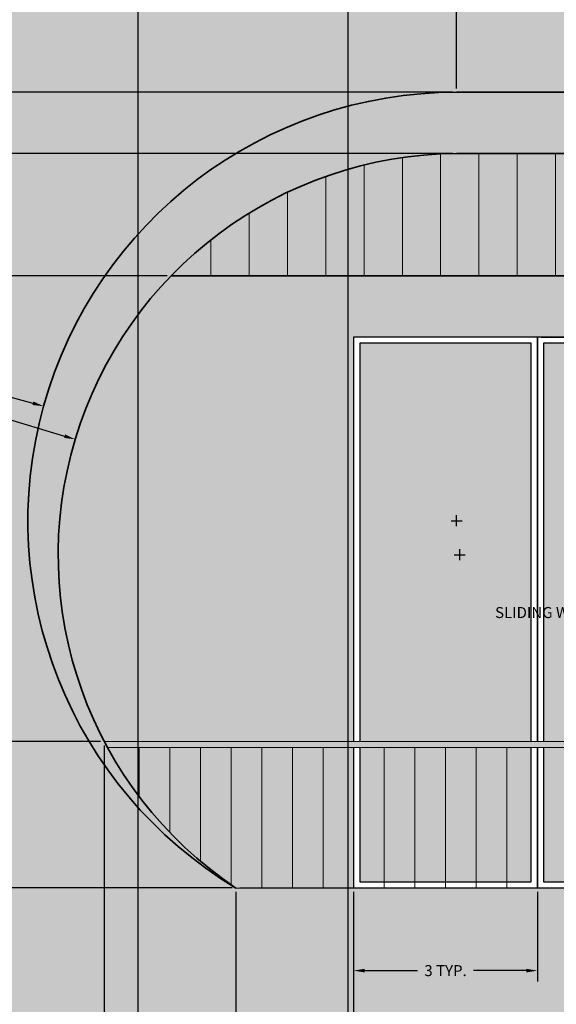
# Model space of a CAD drawing. Units: inches. Extents: x 18 to 59.8, y 2.7 to 81.2.
# Tile 4 of 9: x 26.9 to 35.6, y 29.5 to 45.6. Entities that reach past the tile are written whole.
import ezdxf

# ---------------------------------------------------------------- set-up
doc = ezdxf.new("R2010")
doc.units = ezdxf.units.IN
doc.header["$MEASUREMENT"] = 0
for name, color, linetype, lineweight in [('A-ANNO-DIMS', 2, 'Continuous', 18), ('A-ELEV', 7, 'Continuous', 35), ('A-ELEV-PATT', 8, 'Continuous', 13), ('A-ELEV-RAIL', 7, 'Continuous', 18), ('A-GLAZ', 4, 'Continuous', 25)]:
    doc.layers.add(name, color=color, linetype=linetype, lineweight=lineweight)
doc.styles.get("Standard").update_dxf_attribs({"font": 'arial.ttf'})
doc.dimstyles.get("Standard").update_dxf_attribs({"dimtxt": 0.18, "dimasz": 0.18, "dimexe": 0.18, "dimexo": 0.0625, "dimgap": 0.09, "dimtad": 0, "dimtih": 1, "dimtoh": 1, "dimdec": 1, "dimzin": 0, "dimdsep": 46, "dimlunit": 3, "dimtxsty": 'Standard', "dimcen": 0.09, "dimadec": 0, "dimazin": 0, "dimtfac": 1, "dimtdec": 1, "dimtofl": 0, "dimtmove": 0, "dimatfit": 3, "dimfxl": 1, "dimtolj": 1, "dimtzin": 0, "dimarcsym": 0})

# ---------------------------------------------------------------- blocks, each defined once
blk = doc.blocks.new('WIN-SLIDING-PANEL-1F')
for points in [[(3, 2.393), (3, 9), (0, 9), (0, 2.393)], [(2.9, 2.393), (2.9, 8.9), (0.1, 8.9), (0.1, 2.393)], [(0, 2.293), (0, 0), (3, 0), (3, 2.293)], [(0.1, 2.293), (0.1, 0.1), (2.9, 0.1), (2.9, 2.293)]]:
    blk.add_lwpolyline(points)
blk = doc.blocks.new('*D8')
at = {"layer": 'A-ANNO-DIMS', "color": 0, "lineweight": -2, "transparency": 16777216}
for p, q in [((35.393, 40.441), (36.86, 40.441)), ((36.68, 40.261), (36.68, 36.149)), ((36.68, 31.621), (36.68, 35.733)), ((35.393, 31.441), (36.86, 31.441))]:
    blk.add_line(p, q, dxfattribs=at)
at = {"layer": 'A-ANNO-DIMS', "color": 0, "transparency": 16777216}
for points in [[(36.65, 40.261), (36.71, 40.261), (36.68, 40.441)], [(36.65, 31.621), (36.71, 31.621), (36.68, 31.441)]]:
    blk.add_solid(points, dxfattribs=at)
at = {"layer": 'Defpoints', "color": 0, "transparency": 16777216}
for p in [(35.33, 40.441), (36.68, 40.441), (35.33, 31.441)]:
    blk.add_point(p, dxfattribs=at)
at = {"layer": 'A-ANNO-DIMS', "color": 0, "transparency": 16777216, "insert": (36.68, 35.941), "char_height": 0.18, "attachment_point": 5}
blk.add_mtext('\\A1;SLIDING WINDOW PANEL (1F) 9 TYP.', dxfattribs=at)
blk = doc.blocks.new('*D9')
at = {"layer": 'A-ANNO-DIMS', "color": 0, "lineweight": -2, "transparency": 16777216}
for p, q in [((32.33, 31.378), (32.33, 29.911)), ((35.33, 31.378), (35.33, 29.911)), ((32.51, 30.091), (33.372, 30.091)), ((35.15, 30.091), (34.288, 30.091))]:
    blk.add_line(p, q, dxfattribs=at)
at = {"layer": 'A-ANNO-DIMS', "color": 0, "transparency": 16777216}
for points in [[(32.51, 30.121), (32.51, 30.061), (32.33, 30.091)], [(35.15, 30.121), (35.15, 30.061), (35.33, 30.091)]]:
    blk.add_solid(points, dxfattribs=at)
at = {"layer": 'Defpoints', "color": 0, "transparency": 16777216}
for p in [(32.33, 31.441), (35.33, 31.441), (35.33, 30.091)]:
    blk.add_point(p, dxfattribs=at)
at = {"layer": 'A-ANNO-DIMS', "color": 0, "transparency": 16777216, "insert": (33.83, 30.091), "char_height": 0.18, "attachment_point": 5}
blk.add_mtext('\\A1;3 TYP.', dxfattribs=at)
blk = doc.blocks.new('*D27')
at = {"layer": 'A-ANNO-DIMS', "color": 0, "lineweight": -2, "transparency": 16777216}
for p, q in [((30.469, 31.441), (59.63, 31.441)), ((59.45, 31.261), (59.45, 30.723)), ((59.45, 29.821), (59.45, 30.359)), ((48.922, 29.641), (59.63, 29.641))]:
    blk.add_line(p, q, dxfattribs=at)
at = {"layer": 'A-ANNO-DIMS', "color": 0, "transparency": 16777216}
for points in [[(59.42, 31.261), (59.48, 31.261), (59.45, 31.441)], [(59.42, 29.821), (59.48, 29.821), (59.45, 29.641)]]:
    blk.add_solid(points, dxfattribs=at)
at = {"layer": 'Defpoints', "color": 0, "transparency": 16777216}
for p in [(30.406, 31.441), (48.86, 29.641), (59.45, 29.641)]:
    blk.add_point(p, dxfattribs=at)
at = {"layer": 'A-ANNO-DIMS', "color": 0, "transparency": 16777216, "insert": (59.45, 30.541), "char_height": 0.18, "attachment_point": 5}
blk.add_mtext('\\A1;1.8', dxfattribs=at)
blk = doc.blocks.new('*D50')
at = {"layer": 'A-ANNO-DIMS', "color": 0, "lineweight": -2, "transparency": 16777216}
for p, q in [((33.949, 44.441), (18.09, 44.441)), ((18.27, 44.261), (18.27, 38.123)), ((18.27, 31.621), (18.27, 37.759)), ((30.344, 31.441), (18.09, 31.441))]:
    blk.add_line(p, q, dxfattribs=at)
at = {"layer": 'A-ANNO-DIMS', "color": 0, "transparency": 16777216}
for points in [[(18.24, 44.261), (18.3, 44.261), (18.27, 44.441)], [(18.24, 31.621), (18.3, 31.621), (18.27, 31.441)]]:
    blk.add_solid(points, dxfattribs=at)
at = {"layer": 'Defpoints', "color": 0, "transparency": 16777216}
for p in [(18.27, 44.441), (34.012, 44.441), (30.406, 31.441)]:
    blk.add_point(p, dxfattribs=at)
at = {"layer": 'A-ANNO-DIMS', "color": 0, "transparency": 16777216, "insert": (18.27, 37.941), "char_height": 0.18, "attachment_point": 5}
blk.add_mtext('\\A1;13', dxfattribs=at)
blk = doc.blocks.new('*D51')
at = {"layer": 'A-ANNO-DIMS', "color": 0, "lineweight": -2, "transparency": 16777216}
for p, q in [((34.012, 44.503), (34.012, 81.211)), ((48.86, 43.503), (48.86, 81.211)), ((34.192, 81.031), (40.98, 81.031)), ((48.68, 81.031), (41.891, 81.031))]:
    blk.add_line(p, q, dxfattribs=at)
at = {"layer": 'A-ANNO-DIMS', "color": 0, "transparency": 16777216}
for points in [[(34.192, 81.061), (34.192, 81.001), (34.012, 81.031)], [(48.68, 81.061), (48.68, 81.001), (48.86, 81.031)]]:
    blk.add_solid(points, dxfattribs=at)
at = {"layer": 'Defpoints', "color": 0, "transparency": 16777216}
for p in [(48.86, 81.031), (34.012, 44.441), (48.86, 43.441)]:
    blk.add_point(p, dxfattribs=at)
at = {"layer": 'A-ANNO-DIMS', "color": 0, "transparency": 16777216, "insert": (41.436, 81.031), "char_height": 0.18, "attachment_point": 5}
blk.add_mtext('\\A1;14.848', dxfattribs=at)
blk = doc.blocks.new('*D52')
at = {"layer": 'A-ANNO-DIMS', "color": 0, "lineweight": -2, "transparency": 16777216}
for p, q in [((33.949, 43.441), (18.09, 43.441)), ((18.27, 43.261), (18.27, 42.621)), ((18.27, 41.621), (18.27, 42.26)), ((29.286, 41.441), (18.09, 41.441))]:
    blk.add_line(p, q, dxfattribs=at)
at = {"layer": 'A-ANNO-DIMS', "color": 0, "transparency": 16777216}
for points in [[(18.24, 43.261), (18.3, 43.261), (18.27, 43.441)], [(18.24, 41.621), (18.3, 41.621), (18.27, 41.441)]]:
    blk.add_solid(points, dxfattribs=at)
at = {"layer": 'Defpoints', "color": 0, "transparency": 16777216}
for p in [(18.27, 43.441), (34.012, 43.441), (29.348, 41.441)]:
    blk.add_point(p, dxfattribs=at)
at = {"layer": 'A-ANNO-DIMS', "color": 0, "transparency": 16777216, "insert": (18.27, 42.441), "char_height": 0.18, "attachment_point": 5}
blk.add_mtext('\\A1;2', dxfattribs=at)
blk = doc.blocks.new('*D53')
at = {"layer": 'A-ANNO-DIMS', "color": 0, "lineweight": -2, "transparency": 16777216}
for p, q in [((28.196, 33.834), (18.09, 33.834)), ((18.27, 33.654), (18.27, 32.819)), ((18.27, 31.621), (18.27, 32.455)), ((30.344, 31.441), (18.09, 31.441))]:
    blk.add_line(p, q, dxfattribs=at)
at = {"layer": 'A-ANNO-DIMS', "color": 0, "transparency": 16777216}
for points in [[(18.24, 33.654), (18.3, 33.654), (18.27, 33.834)], [(18.24, 31.621), (18.3, 31.621), (18.27, 31.441)]]:
    blk.add_solid(points, dxfattribs=at)
at = {"layer": 'Defpoints', "color": 0, "transparency": 16777216}
for p in [(28.258, 33.834), (18.27, 31.441), (30.406, 31.441)]:
    blk.add_point(p, dxfattribs=at)
at = {"layer": 'A-ANNO-DIMS', "color": 0, "transparency": 16777216, "insert": (18.27, 32.637), "char_height": 0.18, "attachment_point": 5}
blk.add_mtext('\\A1;2.393', dxfattribs=at)
blk = doc.blocks.new('*D54')
at = {"layer": 'A-ANNO-DIMS', "color": 0, "lineweight": -2, "transparency": 16777216}
for p, q in [((28.258, 33.771), (28.258, 2.671)), ((48.33, 33.352), (48.33, 2.671)), ((28.438, 2.851), (37.899, 2.851)), ((48.15, 2.851), (38.689, 2.851))]:
    blk.add_line(p, q, dxfattribs=at)
at = {"layer": 'A-ANNO-DIMS', "color": 0, "transparency": 16777216}
for points in [[(28.438, 2.881), (28.438, 2.821), (28.258, 2.851)], [(48.15, 2.881), (48.15, 2.821), (48.33, 2.851)]]:
    blk.add_solid(points, dxfattribs=at)
at = {"layer": 'Defpoints', "color": 0, "transparency": 16777216}
for p in [(28.258, 33.834), (48.33, 33.414), (48.33, 2.851)]:
    blk.add_point(p, dxfattribs=at)
at = {"layer": 'A-ANNO-DIMS', "color": 0, "transparency": 16777216, "insert": (38.294, 2.851), "char_height": 0.18, "attachment_point": 5}
blk.add_mtext('\\A1;20.07', dxfattribs=at)
blk = doc.blocks.new('*D56')
at = {"layer": 'A-ANNO-DIMS', "color": 0, "lineweight": -2, "transparency": 16777216}
for p, q in [((30.406, 31.378), (30.406, 2.671)), ((32.33, 31.378), (32.33, 2.671)), ((30.586, 2.851), (30.983, 2.851)), ((32.15, 2.851), (31.753, 2.851))]:
    blk.add_line(p, q, dxfattribs=at)
at = {"layer": 'A-ANNO-DIMS', "color": 0, "transparency": 16777216}
for points in [[(30.586, 2.881), (30.586, 2.821), (30.406, 2.851)], [(32.15, 2.881), (32.15, 2.821), (32.33, 2.851)]]:
    blk.add_solid(points, dxfattribs=at)
at = {"layer": 'Defpoints', "color": 0, "transparency": 16777216}
for p in [(30.406, 31.441), (32.33, 31.441), (32.33, 2.851)]:
    blk.add_point(p, dxfattribs=at)
at = {"layer": 'A-ANNO-DIMS', "color": 0, "transparency": 16777216, "insert": (31.368, 2.851), "char_height": 0.18, "attachment_point": 5}
blk.add_mtext('\\A1;1.924', dxfattribs=at)
blk = doc.blocks.new('*D57')
at = {"layer": 'A-ANNO-DIMS', "color": 0, "lineweight": -2, "transparency": 16777216}
for p, q in [((32.33, 31.378), (32.33, 2.671)), ((44.33, 31.378), (44.33, 2.671)), ((32.51, 2.851), (38.121, 2.851)), ((44.15, 2.851), (38.54, 2.851))]:
    blk.add_line(p, q, dxfattribs=at)
at = {"layer": 'A-ANNO-DIMS', "color": 0, "transparency": 16777216}
for points in [[(32.51, 2.881), (32.51, 2.821), (32.33, 2.851)], [(44.15, 2.881), (44.15, 2.821), (44.33, 2.851)]]:
    blk.add_solid(points, dxfattribs=at)
at = {"layer": 'Defpoints', "color": 0, "transparency": 16777216}
for p in [(32.33, 31.441), (44.33, 31.441), (44.33, 2.851)]:
    blk.add_point(p, dxfattribs=at)
at = {"layer": 'A-ANNO-DIMS', "color": 0, "transparency": 16777216, "insert": (38.33, 2.851), "char_height": 0.18, "attachment_point": 5}
blk.add_mtext('\\A1;12', dxfattribs=at)
blk = doc.blocks.new('*D61')
at = {"layer": 'A-ANNO-DIMS', "color": 0, "lineweight": -2, "transparency": 16777216}
for p, q in [((32.234, 49.378), (32.234, 2.671)), ((47.86, 49.378), (47.86, 2.671)), ((32.414, 2.851), (39.592, 2.851)), ((47.68, 2.851), (40.502, 2.851))]:
    blk.add_line(p, q, dxfattribs=at)
at = {"layer": 'A-ANNO-DIMS', "color": 0, "transparency": 16777216}
for points in [[(32.414, 2.881), (32.414, 2.821), (32.234, 2.851)], [(47.68, 2.881), (47.68, 2.821), (47.86, 2.851)]]:
    blk.add_solid(points, dxfattribs=at)
at = {"layer": 'Defpoints', "color": 0, "transparency": 16777216}
for p in [(32.234, 49.441), (47.86, 49.441), (47.86, 2.851)]:
    blk.add_point(p, dxfattribs=at)
at = {"layer": 'A-ANNO-DIMS', "color": 0, "transparency": 16777216, "insert": (40.047, 2.851), "char_height": 0.18, "attachment_point": 5}
blk.add_mtext('\\A1;15.626', dxfattribs=at)
blk = doc.blocks.new('*D66')
at = {"layer": 'A-ANNO-DIMS', "color": 0, "lineweight": -2, "transparency": 16777216}
for p, q in [((28.804, 51.378), (28.804, 2.671)), ((48.567, 51.179), (48.567, 2.671)), ((28.984, 2.851), (38.231, 2.851)), ((48.387, 2.851), (39.14, 2.851))]:
    blk.add_line(p, q, dxfattribs=at)
at = {"layer": 'A-ANNO-DIMS', "color": 0, "transparency": 16777216}
for points in [[(28.984, 2.881), (28.984, 2.821), (28.804, 2.851)], [(48.387, 2.881), (48.387, 2.821), (48.567, 2.851)]]:
    blk.add_solid(points, dxfattribs=at)
at = {"layer": 'Defpoints', "color": 0, "transparency": 16777216}
for p in [(28.804, 51.441), (48.567, 51.242), (48.567, 2.851)]:
    blk.add_point(p, dxfattribs=at)
at = {"layer": 'A-ANNO-DIMS', "color": 0, "transparency": 16777216, "insert": (38.685, 2.851), "char_height": 0.18, "attachment_point": 5}
blk.add_mtext('\\A1;19.764', dxfattribs=at)
blk = doc.blocks.new('*D69')
at = {"layer": 'A-ANNO-DIMS', "color": 0, "lineweight": -2, "transparency": 16777216}
for p, q in [((23.039, 40.435), (23.219, 40.435)), ((23.219, 40.435), (27.093, 39.36)), ((34.012, 37.351), (34.012, 37.531)), ((33.922, 37.441), (34.102, 37.441))]:
    blk.add_line(p, q, dxfattribs=at)
at = {"layer": 'A-ANNO-DIMS', "color": 0, "transparency": 16777216}
blk.add_solid([(27.101, 39.389), (27.085, 39.331), (27.266, 39.312)], dxfattribs=at)
at = {"layer": 'Defpoints', "color": 0, "transparency": 16777216}
for p in [(27.266, 39.312), (34.012, 37.441)]:
    blk.add_point(p, dxfattribs=at)
at = {"layer": 'A-ANNO-DIMS', "color": 0, "transparency": 16777216, "insert": (22.804, 40.435), "char_height": 0.18, "attachment_point": 5}
blk.add_mtext('\\A1;R7', dxfattribs=at)
blk = doc.blocks.new('*D70')
at = {"layer": 'A-ANNO-DIMS', "color": 0, "lineweight": -2, "transparency": 16777216}
for p, q in [((23.835, 39.903), (24.015, 39.903)), ((24.015, 39.903), (27.611, 38.823)), ((33.973, 36.884), (34.153, 36.884)), ((34.063, 36.794), (34.063, 36.974))]:
    blk.add_line(p, q, dxfattribs=at)
at = {"layer": 'A-ANNO-DIMS', "color": 0, "transparency": 16777216}
blk.add_solid([(27.619, 38.851), (27.602, 38.794), (27.783, 38.771)], dxfattribs=at)
at = {"layer": 'Defpoints', "color": 0, "transparency": 16777216}
for p in [(27.783, 38.771), (34.063, 36.884)]:
    blk.add_point(p, dxfattribs=at)
at = {"layer": 'A-ANNO-DIMS', "color": 0, "transparency": 16777216, "insert": (23.355, 39.903), "char_height": 0.18, "attachment_point": 5}
blk.add_mtext('\\A1;R6.557', dxfattribs=at)

msp = doc.modelspace()

# ---------------------------------------------------------------- hatches: boundary and pattern name
at = {"layer": 'A-ELEV-PATT'}
h = msp.add_hatch(color=256, dxfattribs=at)
h.set_gradient(color1=(255, 255, 255), color2=(199, 200, 202))
h.paths.add_polyline_path([(38.86, 75.4521, 0.4125527), (36.86, 77.4407), (21.86, 77.4407), (21.86, 22.4407), (22.86, 22.4407), (48.86, 22.4407), (48.86, 30.9234, 0.4074473), (48.3302, 31.4407), (30.4061, 31.4407, -0.7603989), (34.0116, 44.4407), (47.86, 44.4407, -0.4142136), (48.86, 43.4407), (48.86, 48.4407, 0.4142136), (47.86, 49.4407), (32.2338, 49.4407, -0.2243142), (27.8411, 52.8427, -0.8480129), (38.86, 61.4407)])
h.paths.add_polyline_path([(55.86, 77.4407), (54.86, 77.4407), (54.86, 22.2407), (55.86, 22.2407)])
h.paths.add_polyline_path([(54.86, 51.5407), (53.4401, 51.5407), (53.4401, 29.6407), (54.86, 29.6407)])
h.paths.add_polyline_path([(54.86, 61.4407), (53.4401, 57.4407), (53.4401, 51.6407), (54.86, 51.6407)])
h.paths.add_polyline_path([(54.86, 29.4407), (54.471, 29.4407), (54.471, 22.2407), (54.86, 22.2407)])
h.paths.add_polyline_path([(55.5745, 22.2407), (54.86, 22.2407), (54.5745, 22.2407), (53.9347, 21.7925), (54.5877, 21.5495)])
h.paths.add_polyline_path([(54.5991, 21.5452), (53.9443, 21.789), (53.9443, 18.4407), (54.5991, 18.4407)])
h.paths.add_polyline_path([(53.9443, 21.789), (53.9347, 21.7925), (53.5816, 21.5452), (53.5816, 18.4407), (53.9443, 18.4407)])
h.paths.add_polyline_path([(53.3648, 20.6928), (52.8956, 21.0646), (52.8956, 18.4407), (53.3648, 18.4407)])
h.paths.add_polyline_path([(52.8956, 21.0646), (50.5775, 19.4407), (50.5775, 18.4407), (52.8956, 18.4407)])
h.paths.add_polyline_path([(53.5816, 21.5452), (52.8956, 21.0646), (53.3648, 20.6928), (53.5816, 20.8447)])
h.paths.add_polyline_path([(26.8109, 19.4407), (24.9672, 20.8407), (24.9672, 18.4407), (26.8109, 18.4407)])
h.paths.add_polyline_path([(24.9672, 20.8407), (24.4165, 20.8427), (24.4165, 18.4407), (24.9672, 18.4407)])
h.paths.add_polyline_path([(24.4165, 20.8427), (24.4165, 21.2589), (24.0588, 21.5305), (24.0301, 21.5183), (24.0301, 18.4407), (24.4165, 18.4407)])
h.paths.add_polyline_path([(24.0301, 21.5183), (23.4165, 21.2589), (23.4165, 18.4407), (24.0301, 18.4407)])
h.paths.add_polyline_path([(24.0301, 21.5183), (24.0588, 21.5305), (23.1234, 22.2407), (22.1234, 22.2407), (23.4165, 21.2589)])
h.paths.add_polyline_path([(24.4165, 21.2589), (24.4165, 20.8427), (24.9672, 20.8407)])
h.paths.add_polyline_path([(47.86, 18.4407), (29.86, 18.4407), (29.86, 6.4407), (30.86, 6.4407), (30.86, 17.4407), (38.86, 17.4407), (46.86, 17.4407), (46.86, 6.4407), (47.86, 6.4407)])
h.paths.add_polyline_path([(54.5756, 15.215), (54.5756, 6.4407), (55.86, 6.4407), (55.86, 18.4407), (47.86, 18.4407), (47.86, 6.4407), (49.1482, 6.4407), (49.1482, 15.215, -1)])
h = msp.add_hatch(color=256, dxfattribs=at)
h.paths.add_polyline_path([(27.8411, 52.8427, -0.7443789), (36.86, 61.4407), (38.86, 61.4407, 0.8480129)])
h.paths.add_polyline_path([(47.86, 44.4407), (34.0116, 44.4407, 0.7603989), (30.4061, 31.4407, -0.7376246), (34.0116, 43.4407), (47.86, 43.4407, -0.4142136), (48.86, 42.4407), (48.86, 43.4407, 0.4142136)])
h.paths.add_polyline_path([(54.5756, 15.215), (54.5756, 6.4407), (55.86, 6.4407), (55.86, 18.4407), (47.86, 18.4407), (47.86, 6.4407), (49.1482, 6.4407), (49.1482, 15.215, -1)])
h.paths.add_polyline_path([(47.86, 18.4407), (29.86, 18.4407), (29.86, 6.4407), (30.86, 6.4407), (30.86, 17.4407), (38.86, 17.4407), (46.86, 17.4407), (46.86, 6.4407), (47.86, 6.4407)])
h.paths.add_polyline_path([(55.86, 77.4407), (54.86, 77.4407), (54.86, 22.2407), (55.86, 22.2407)])
h = msp.add_hatch(color=256, dxfattribs=at)
h.dxf.hatch_style = 1
h.paths.add_polyline_path([(54.86, 69.4407), (38.86, 69.4407), (38.86, 61.4407), (54.86, 61.4407)])
h.paths.add_polyline_path([(54.86, 61.4407), (38.86, 61.4407), (36.86, 61.4407, 0.443414), (27.6986, 58.4407), (48.86, 58.4407), (48.86, 57.4407), (53.4401, 57.4407)])
h.paths.add_polyline_path([(37.4994, 59.9399), (37.4994, 59.8198, -2.4106499), (37.1187, 59.8198), (37.1187, 59.9399)], flags=16)
h.paths.add_polyline_path([(42.6125, 59.8012), (42.6125, 59.9213), (42.9933, 59.9213), (42.9933, 59.8012, -2.4106499)], flags=16)
h.paths.add_polyline_path([(49.5965, 59.971), (49.5965, 60.091), (49.9773, 60.091), (49.9773, 59.971, -2.4106499)], flags=16)
h.paths.add_polyline_path([(44.4671, 57.0407), (32.6671, 57.0407), (32.6671, 56.0407), (44.4671, 56.0407)])
h.paths.add_polyline_path([(47.86, 43.4407), (46.86, 43.4407), (34.0116, 43.4407, 0.2012983), (29.3481, 41.4407), (47.86, 41.4407, 1)])
h.paths.add_polyline_path([(36.5542, 42.5145), (36.5542, 42.6346), (36.9349, 42.6346), (36.9349, 42.5145, -2.4106499)], flags=16)
h.paths.add_polyline_path([(42.939, 42.5402), (42.939, 42.6603), (43.3198, 42.6603), (43.3198, 42.5402, -2.4106499)], flags=16)
h.paths.add_polyline_path([(54.471, 29.4407), (48.86, 29.4407), (48.86, 22.2407), (54.471, 22.2407)])
h.paths.add_polyline_path([(54.5745, 22.2407), (23.1234, 22.2407), (26.8109, 19.4407), (50.5775, 19.4407)])
h.paths.add_polyline_path([(54.5756, 15.215, 1), (49.1482, 15.215), (49.1482, 6.4407), (54.5756, 6.4407)])
h.paths.add_polyline_path([(49.8323, 12.602), (49.8323, 9.1225), (49.6657, 9.1225), (49.6657, 12.602)], flags=16)
h = msp.add_hatch(dxfattribs=at)
h.set_pattern_fill('ANSI31', color=256, scale=5, angle=45, style=0)
h.paths.add_polyline_path([(54.86, 69.4407), (38.86, 69.4407), (38.86, 61.4407), (54.86, 61.4407)])
h.paths.add_polyline_path([(54.86, 61.4407), (38.86, 61.4407), (36.86, 61.4407, 0.443414), (27.6986, 58.4407), (48.86, 58.4407), (48.86, 57.4407), (53.4401, 57.4407)])
h.paths.add_polyline_path([(37.1661, 59.8577), (37.1187, 59.8577), (37.1187, 59.9399), (37.4994, 59.9399), (37.4994, 59.8577), (37.452, 59.8577, -3.476462)], flags=16)
h.paths.add_polyline_path([(42.66, 59.8391), (42.6125, 59.8391), (42.6125, 59.9213), (42.9933, 59.9213), (42.9933, 59.8391), (42.9458, 59.8391, -3.476462)], flags=16)
h.paths.add_polyline_path([(49.644, 60.0088), (49.5965, 60.0088), (49.5965, 60.091), (49.9773, 60.091), (49.9773, 60.0088), (49.9298, 60.0088, -3.476462)], flags=16)
h.paths.add_polyline_path([(44.4671, 57.0407), (32.6671, 57.0407), (32.6671, 56.0407), (44.4671, 56.0407)])
h.paths.add_polyline_path([(47.86, 43.4407), (46.86, 43.4407), (34.0116, 43.4407, 0.2012983), (29.3481, 41.4407), (47.86, 41.4407, 1)])
h.paths.add_polyline_path([(36.6016, 42.5524), (36.5542, 42.5524), (36.5542, 42.6346), (36.9349, 42.6346), (36.9349, 42.5524), (36.8875, 42.5524, -3.476462)], flags=16)
h.paths.add_polyline_path([(42.9865, 42.578), (42.939, 42.578), (42.939, 42.6603), (43.3198, 42.6603), (43.3198, 42.578), (43.2723, 42.578, -3.476462)], flags=16)
h.paths.add_polyline_path([(54.471, 29.4407), (48.86, 29.4407), (48.86, 22.2407), (54.471, 22.2407)])
h.paths.add_polyline_path([(54.5745, 22.2407), (23.1234, 22.2407), (26.8109, 19.4407), (50.5775, 19.4407)])
h.paths.add_polyline_path([(54.5756, 15.215, 1), (49.1482, 15.215), (49.1482, 6.4407), (54.5756, 6.4407)])
h.paths.add_polyline_path([(49.8323, 9.1225), (49.6657, 9.1225), (49.6657, 12.602), (49.8323, 12.602)], flags=16)
at = {"layer": 'A-ELEV-PATT', "transparency": 33554620}
h = msp.add_hatch(color=256, dxfattribs=at)
h.set_gradient(color1=(147, 149, 152))
edge = h.paths.add_edge_path()
edge.add_line((32.5671, 55.9407), (32.5671, 57.1407))
edge.add_line((32.5671, 57.1407), (44.5671, 57.1407))
edge.add_line((44.5671, 57.1407), (44.5671, 55.9407))
edge.add_line((44.5671, 55.9407), (44.5671, 51.5407))
edge.add_line((44.5671, 51.5407), (47.9208, 51.5407))
edge.add_spline(control_points=[(47.9208, 51.5407), (48.1524, 51.5145), (48.3597, 51.3781), (48.5671, 51.2416)], knot_values=[0, 0, 0, 0, 0.7121901, 0.7121901, 0.7121901, 0.7121901], degree=3, periodic=0)
edge.add_line((48.5671, 51.2416), (48.5671, 49.1479))
edge.add_arc((47.86, 48.4407), 1, 5.73917, 45, ccw=False)
edge.add_line((48.855, 48.5407), (48.86, 48.5407))
edge.add_line((48.86, 48.5407), (48.86, 49.4407))
edge.add_line((48.86, 49.4407), (48.86, 58.4407))
edge.add_line((48.86, 58.4407), (27.6986, 58.4407))
edge.add_arc((33.6382, 55.7911), 6.5038, 155.95802, 220.80748)
edge.add_line((28.7154, 51.5407), (32.5671, 51.5407))
edge.add_line((32.5671, 51.5407), (32.5671, 55.9407))
edge = h.paths.add_edge_path()
edge.add_line((32.3302, 40.4407), (35.3302, 40.4407))
edge.add_line((35.3302, 40.4407), (38.3302, 40.4407))
edge.add_line((38.3302, 40.4407), (41.3302, 40.4407))
edge.add_line((41.3302, 40.4407), (44.3302, 40.4407))
edge.add_line((44.3302, 40.4407), (44.3302, 33.8336))
edge.add_line((44.3302, 33.8336), (47.6839, 33.8336))
edge.add_spline(control_points=[(47.6839, 33.8336), (47.9155, 33.8074), (48.1229, 33.671), (48.3302, 33.5345)], knot_values=[0, 0, 0, 0, 0.7121901, 0.7121901, 0.7121901, 0.7121901], degree=3, periodic=0)
edge.add_line((48.3302, 33.5345), (48.3302, 31.4407))
edge.add_arc((48.3304, 30.911), 0.5297, 1.3425, 90.01573, ccw=False)
edge.add_line((48.86, 30.9234), (48.86, 38.6846))
edge.add_line((48.86, 38.6846), (50.793, 38.6846))
edge.add_line((50.793, 38.6846), (50.793, 41.316))
edge.add_line((50.793, 41.316), (52.927, 41.316))
edge.add_line((52.927, 41.316), (52.927, 38.6846))
edge.add_line((52.927, 38.6846), (53.4401, 38.6846))
edge.add_line((53.4401, 38.6846), (53.4401, 48.4407))
edge.add_line((53.4401, 48.4407), (48.86, 48.4407))
edge.add_line((48.86, 48.4407), (48.86, 42.4407))
edge.add_arc((47.86, 42.4407), 1, -90, 0, ccw=False)
edge.add_line((47.86, 41.4407), (29.3481, 41.4407))
edge.add_arc((34.0631, 36.8836), 6.5573, 135.97541, 207.71831)
edge.add_line((28.2583, 33.8336), (32.3302, 33.8336))
edge.add_line((32.3302, 33.8336), (32.3302, 40.4407))
h.paths.add_polyline_path([(53.4401, 57.4407), (48.86, 57.4407), (48.86, 51.6407), (53.4401, 51.6407)])
h.paths.add_polyline_path([(29.5671, 51.4407), (28.8035, 51.4407, 0.040451), (29.5671, 50.7191)], flags=17)
h.paths.add_polyline_path([(30.0671, 51.4407), (29.5671, 51.4407), (29.5671, 50.7191, 0.0237787), (30.0671, 50.3554)], flags=17)
h.paths.add_polyline_path([(30.5671, 51.4407), (30.0671, 51.4407), (30.0671, 50.3554, 0.0223729), (30.5671, 50.0581)], flags=17)
h.paths.add_polyline_path([(31.0671, 51.4407), (30.5671, 51.4407), (30.5671, 50.0581, 0.021345), (31.0671, 49.8171)], flags=17)
h.paths.add_polyline_path([(31.5671, 51.4407), (31.0671, 51.4407), (31.0671, 49.8171, 0.0205858), (31.5671, 49.6259)], flags=17)
h.paths.add_polyline_path([(32.0671, 51.4407), (31.5671, 51.4407), (31.5671, 49.6259, 0.0200299), (32.0671, 49.4799)], flags=17)
h.paths.add_polyline_path([(32.5671, 51.4407), (32.0671, 51.4407), (32.0671, 49.4799, 0.0065845), (32.2338, 49.4407), (32.5671, 49.4407)], flags=17)
h.paths.add_polyline_path([(45.0671, 51.4407), (44.5671, 51.4407), (44.5671, 49.4407), (45.0671, 49.4407)], flags=17)
h.paths.add_polyline_path([(45.5671, 51.4407), (45.0671, 51.4407), (45.0671, 49.4407), (45.5671, 49.4407)], flags=17)
h.paths.add_polyline_path([(46.0671, 51.4407), (45.5671, 51.4407), (45.5671, 49.4407), (46.0671, 49.4407)], flags=17)
h.paths.add_polyline_path([(46.5671, 51.4407), (46.0671, 51.4407), (46.0671, 49.4407), (46.5671, 49.4407)], flags=17)
h.paths.add_polyline_path([(47.0671, 51.4407), (46.5671, 51.4407), (46.5671, 49.4407), (47.0671, 49.4407)], flags=17)
h.paths.add_polyline_path([(47.5671, 51.4407), (47.0671, 51.4407), (47.0671, 49.4407), (47.5671, 49.4407)], flags=17)
edge = h.paths.add_edge_path(flags=17)
edge.add_spline(control_points=[(48.0671, 51.4184), (48.0217, 51.4311), (47.9752, 51.4389), (47.9273, 51.4407)], knot_values=[0.570104, 0.570104, 0.570104, 0.570104, 0.7151116, 0.7151116, 0.7151116, 0.7151116], degree=3, periodic=0)
edge.add_line((47.9273, 51.4407), (47.5671, 51.4407))
edge.add_line((47.5671, 51.4407), (47.5671, 49.4407))
edge.add_line((47.5671, 49.4407), (47.86, 49.4407))
edge.add_arc((47.86, 48.4407), 1, 78.04714, 90, ccw=False)
edge.add_line((48.0671, 49.4191), (48.0671, 51.4184))
edge = h.paths.add_edge_path(flags=17)
edge.add_spline(control_points=[(48.5671, 51.1212), (48.4062, 51.2449), (48.2454, 51.3687), (48.0671, 51.4184)], knot_values=[0, 0, 0, 0, 0.570104, 0.570104, 0.570104, 0.570104], degree=3, periodic=0)
edge.add_line((48.0671, 51.4184), (48.0671, 49.4191))
edge.add_arc((47.86, 48.4407), 1, 45, 78.04714, ccw=False)
edge.add_line((48.5671, 49.1479), (48.5671, 51.1212))
h.paths.add_polyline_path([(49.36, 51.5407), (48.86, 51.5407), (48.86, 49.4407), (48.86, 48.5407), (49.36, 48.5407)])
h.paths.add_polyline_path([(49.86, 51.5407), (49.36, 51.5407), (49.36, 48.5407), (49.86, 48.5407)])
h.paths.add_polyline_path([(50.36, 51.5407), (49.86, 51.5407), (49.86, 48.5407), (50.36, 48.5407)])
h.paths.add_polyline_path([(50.86, 51.5407), (50.36, 51.5407), (50.36, 48.5407), (50.86, 48.5407)])
h.paths.add_polyline_path([(51.36, 51.5407), (50.86, 51.5407), (50.86, 48.5407), (51.36, 48.5407)])
h.paths.add_polyline_path([(51.86, 51.5407), (51.36, 51.5407), (51.36, 48.5407), (51.86, 48.5407)])
h.paths.add_polyline_path([(52.36, 51.5407), (51.86, 51.5407), (51.86, 48.5407), (52.36, 48.5407)])
h.paths.add_polyline_path([(52.86, 51.5407), (52.36, 51.5407), (52.36, 48.5407), (52.86, 48.5407)])
h.paths.add_polyline_path([(53.36, 51.5407), (52.86, 51.5407), (52.86, 48.5407), (53.36, 48.5407)])
h.paths.add_polyline_path([(53.4401, 38.6846), (48.86, 38.6846), (48.86, 30.9234), (48.86, 29.6407), (53.4401, 29.6407)])
h.paths.add_polyline_path([(28.8302, 33.7336), (28.3119, 33.7336, 0.0364452), (28.8302, 32.9319)], flags=17)
h.paths.add_polyline_path([(29.3302, 33.7336), (28.8302, 33.7336), (28.8302, 32.9319, 0.0294201), (29.3302, 32.3451)], flags=17)
h.paths.add_polyline_path([(29.8302, 33.7336), (29.3302, 33.7336), (29.3302, 32.3451, 0.0261691), (29.8302, 31.8755)], flags=17)
h.paths.add_polyline_path([(30.3302, 33.7336), (29.8302, 33.7336), (29.8302, 31.8755, 0.0240263), (30.3302, 31.4925)], flags=17)
h.paths.add_polyline_path([(30.8302, 33.7336), (30.3302, 33.7336), (30.3302, 31.4925, 0.0035006), (30.4061, 31.4407), (30.8302, 31.4407)], flags=17)
h.paths.add_polyline_path([(31.3302, 33.7336), (30.8302, 33.7336), (30.8302, 31.4407), (31.3302, 31.4407)], flags=17)
h.paths.add_polyline_path([(31.8302, 33.7336), (31.3302, 33.7336), (31.3302, 31.4407), (31.8302, 31.4407)], flags=17)
h.paths.add_polyline_path([(32.3302, 33.7336), (31.8302, 33.7336), (31.8302, 31.4407), (32.3302, 31.4407)], flags=17)
h.paths.add_polyline_path([(44.8302, 33.7336), (44.3302, 33.7336), (44.3302, 31.4407), (44.8302, 31.4407)], flags=17)
h.paths.add_polyline_path([(45.3302, 33.7336), (44.8302, 33.7336), (44.8302, 31.4407), (45.3302, 31.4407)], flags=17)
h.paths.add_polyline_path([(45.8302, 33.7336), (45.3302, 33.7336), (45.3302, 31.4407), (45.8302, 31.4407)], flags=17)
h.paths.add_polyline_path([(46.3302, 33.7336), (45.8302, 33.7336), (45.8302, 31.4407), (46.3302, 31.4407)], flags=17)
h.paths.add_polyline_path([(46.8302, 33.7336), (46.3302, 33.7336), (46.3302, 31.4407), (46.8302, 31.4407)], flags=17)
h.paths.add_polyline_path([(47.3302, 33.7336), (46.8302, 33.7336), (46.8302, 31.4407), (47.3302, 31.4407)], flags=17)
edge = h.paths.add_edge_path(flags=16)
edge.add_spline(control_points=[(47.8302, 33.7113), (47.7849, 33.7239), (47.7384, 33.7318), (47.6905, 33.7336)], knot_values=[0.570104, 0.570104, 0.570104, 0.570104, 0.7151116, 0.7151116, 0.7151116, 0.7151116], degree=3, periodic=0)
edge.add_line((47.6905, 33.7336), (47.3302, 33.7336))
edge.add_line((47.3302, 33.7336), (47.3302, 31.4407))
edge.add_line((47.3302, 31.4407), (47.8302, 31.4407))
edge.add_line((47.8302, 31.4407), (47.8302, 33.7113))
h.paths.add_polyline_path([(48.86, 38.6846), (50.793, 38.6846), (50.793, 41.316), (52.927, 41.316), (52.927, 38.6846), (53.4401, 38.6846), (53.4401, 48.4407), (48.86, 48.4407), (48.86, 42.4407, -0.4142136), (47.86, 41.4407), (29.3481, 41.4407, 0.3236799), (28.2583, 33.8336), (32.3302, 33.8336), (32.3302, 40.4407), (35.3302, 40.4407), (38.3302, 40.4407), (41.3302, 40.4407), (44.3302, 40.4407), (44.3302, 33.8336), (28.2583, 33.8336, 0.0043267), (28.3119, 33.7336), (28.8302, 33.7336), (29.3302, 33.7336), (29.8302, 33.7336), (30.3302, 33.7336), (30.8302, 33.7336), (31.3302, 33.7336), (31.8302, 33.7336), (32.3302, 33.7336), (47.3302, 33.7336), (47.3302, 31.4407), (47.8302, 31.4407), (48.3302, 31.4407, -0.4074473), (48.86, 30.9234)])
edge = h.paths.add_edge_path(flags=0)
edge.add_spline(control_points=[(47.8302, 33.7113), (47.7849, 33.7239), (47.7384, 33.7318), (47.6905, 33.7336)], knot_values=[0.570104, 0.570104, 0.570104, 0.570104, 0.7151116, 0.7151116, 0.7151116, 0.7151116], degree=3, periodic=0)
edge.add_line((47.6905, 33.7336), (47.3302, 33.7336))
edge.add_line((47.3302, 33.7336), (47.3302, 31.4407))
edge.add_line((47.3302, 31.4407), (47.8302, 31.4407))
edge.add_line((47.8302, 31.4407), (47.8302, 33.7113))
h = msp.add_hatch(color=256, dxfattribs=at)
h.set_gradient(color1=(147, 149, 152))
edge = h.paths.add_edge_path()
edge.add_line((44.3302, 33.8336), (47.6839, 33.8336))
edge.add_spline(control_points=[(47.6839, 33.8336), (47.9155, 33.8074), (48.1229, 33.671), (48.3302, 33.5345)], knot_values=[0, 0, 0, 0, 0.7121901, 0.7121901, 0.7121901, 0.7121901], degree=3, periodic=0)
edge.add_line((48.3302, 33.5345), (48.3302, 31.4407))
edge.add_arc((48.3304, 30.911), 0.5297, 1.3425, 90.01573, ccw=False)
edge.add_line((48.86, 30.9234), (48.86, 38.6846))
edge.add_line((48.86, 38.6846), (50.793, 38.6846))
edge.add_line((50.793, 38.6846), (50.793, 41.316))
edge.add_line((50.793, 41.316), (52.927, 41.316))
edge.add_line((52.927, 41.316), (52.927, 38.6846))
edge.add_line((52.927, 38.6846), (53.4401, 38.6846))
edge.add_line((53.4401, 38.6846), (53.4401, 48.4407))
edge.add_line((53.4401, 48.4407), (48.86, 48.4407))
edge.add_line((48.86, 48.4407), (48.86, 42.4407))
edge.add_arc((47.86, 42.4407), 1, -90, 0, ccw=False)
edge.add_line((47.86, 41.4407), (29.3481, 41.4407))
edge.add_arc((34.0631, 36.8836), 6.5573, 135.97541, 207.71831)
edge.add_line((28.2583, 33.8336), (32.3302, 33.8336))
edge.add_line((32.3302, 33.8336), (32.3302, 40.4407))
edge.add_line((32.3302, 40.4407), (35.3302, 40.4407))
edge.add_line((35.3302, 40.4407), (38.3302, 40.4407))
edge.add_line((38.3302, 40.4407), (41.3302, 40.4407))
edge.add_line((41.3302, 40.4407), (44.3302, 40.4407))
edge.add_line((44.3302, 40.4407), (44.3302, 33.8336))
h = msp.add_hatch(color=256, dxfattribs=at)
h.set_gradient(color1=(173, 221, 247))
h.paths.add_polyline_path([(35.2302, 40.3407), (32.4302, 40.3407), (32.4302, 33.8336), (35.2302, 33.8336)])
h.paths.add_polyline_path([(32.8302, 33.7336), (32.4302, 33.7336), (32.4302, 31.5407), (32.8302, 31.5407)])
h.paths.add_polyline_path([(33.3302, 33.7336), (32.8302, 33.7336), (32.8302, 31.5407), (33.3302, 31.5407)])
h.paths.add_polyline_path([(33.8302, 33.7336), (33.3302, 33.7336), (33.3302, 31.5407), (33.8302, 31.5407)])
h.paths.add_polyline_path([(34.3302, 33.7336), (33.8302, 33.7336), (33.8302, 31.5407), (34.3302, 31.5407)])
h.paths.add_polyline_path([(34.8302, 33.7336), (34.3302, 33.7336), (34.3302, 31.5407), (34.8302, 31.5407)])
h.paths.add_polyline_path([(35.2302, 33.7336), (34.8302, 33.7336), (34.8302, 31.5407), (35.2302, 31.5407)])
h.paths.add_polyline_path([(38.2302, 40.3407), (35.4302, 40.3407), (35.4302, 33.8336), (38.2302, 33.8336)])
h.paths.add_polyline_path([(35.8302, 33.7336), (35.4302, 33.7336), (35.4302, 31.5407), (35.8302, 31.5407)])
h.paths.add_polyline_path([(36.3302, 33.7336), (35.8302, 33.7336), (35.8302, 31.5407), (36.3302, 31.5407)])
h.paths.add_polyline_path([(36.8302, 33.7336), (36.3302, 33.7336), (36.3302, 31.5407), (36.8302, 31.5407)])
h.paths.add_polyline_path([(37.3302, 33.7336), (36.8302, 33.7336), (36.8302, 31.5407), (37.3302, 31.5407)])
h.paths.add_polyline_path([(37.8302, 33.7336), (37.3302, 33.7336), (37.3302, 31.5407), (37.8302, 31.5407)])
h.paths.add_polyline_path([(38.2302, 33.7336), (37.8302, 33.7336), (37.8302, 31.5407), (38.2302, 31.5407)])
h.paths.add_polyline_path([(41.2302, 40.3407), (38.4302, 40.3407), (38.4302, 33.8336), (41.2302, 33.8336)])
h.paths.add_polyline_path([(44.2302, 40.3407), (41.4302, 40.3407), (41.4302, 33.8336), (44.2302, 33.8336)])
h.paths.add_polyline_path([(38.8302, 33.7336), (38.4302, 33.7336), (38.4302, 31.5407), (38.8302, 31.5407)])
h.paths.add_polyline_path([(39.3302, 33.7336), (38.8302, 33.7336), (38.8302, 31.5407), (39.3302, 31.5407)])
h.paths.add_polyline_path([(39.8302, 33.7336), (39.3302, 33.7336), (39.3302, 31.5407), (39.8302, 31.5407)])
h.paths.add_polyline_path([(40.3302, 33.7336), (39.8302, 33.7336), (39.8302, 31.5407), (40.3302, 31.5407)])
h.paths.add_polyline_path([(40.8302, 33.7336), (40.3302, 33.7336), (40.3302, 31.5407), (40.8302, 31.5407)])
h.paths.add_polyline_path([(41.2302, 33.7336), (40.8302, 33.7336), (40.8302, 31.5407), (41.2302, 31.5407)])
h.paths.add_polyline_path([(41.8302, 33.7336), (41.4302, 33.7336), (41.4302, 31.5407), (41.8302, 31.5407)])
h.paths.add_polyline_path([(42.3302, 33.7336), (41.8302, 33.7336), (41.8302, 31.5407), (42.3302, 31.5407)])
h.paths.add_polyline_path([(42.8302, 33.7336), (42.3302, 33.7336), (42.3302, 31.5407), (42.8302, 31.5407)])
h.paths.add_polyline_path([(43.3302, 33.7336), (42.8302, 33.7336), (42.8302, 31.5407), (43.3302, 31.5407)])
h.paths.add_polyline_path([(43.8302, 33.7336), (43.3302, 33.7336), (43.3302, 31.5407), (43.8302, 31.5407)])
h.paths.add_polyline_path([(44.2302, 33.7336), (43.8302, 33.7336), (43.8302, 31.5407), (44.2302, 31.5407)])
at = {"layer": 'A-ELEV-PATT'}
h = msp.add_hatch(color=256, dxfattribs=at)
h.paths.add_polyline_path([(38.86, 17.4407), (30.86, 17.4407), (30.86, 6.4407), (30.96, 6.4407), (30.96, 17.3407), (38.86, 17.3407)])
h.paths.add_polyline_path([(46.86, 17.4407), (38.86, 17.4407), (38.86, 17.3407), (46.76, 17.3407), (46.76, 6.4407), (46.86, 6.4407)])
h.paths.add_polyline_path([(49.8323, 12.602), (49.6657, 12.602), (49.6657, 9.1225), (49.8323, 9.1225)])
h.paths.add_polyline_path([(48.86, 22.4407), (21.86, 22.4407), (21.86, 22.2407), (48.86, 22.2407)])
h.paths.add_polyline_path([(54.86, 29.6407), (48.86, 29.6407), (48.86, 29.4407), (54.86, 29.4407)])
edge = h.paths.add_edge_path()
edge.add_spline(control_points=[(48.3302, 33.5345), (48.1229, 33.671), (47.9155, 33.8074), (47.6839, 33.8336)], knot_values=[0, 0, 0, 0, 0.7121901, 0.7121901, 0.7121901, 0.7121901], degree=3, periodic=0)
edge.add_line((47.6839, 33.8336), (28.2583, 33.8336))
edge.add_arc((34.0631, 36.8836), 6.5573, 207.71831, 208.7099)
edge.add_line((28.3119, 33.7336), (47.6238, 33.7336))
edge.add_spline(control_points=[(47.6238, 33.7336), (47.6461, 33.7341), (47.6685, 33.7345), (47.6905, 33.7336)], knot_values=[0, 0, 0, 0, 0.0667446, 0.0667446, 0.0667446, 0.0667446], degree=3, periodic=0)
edge.add_spline(control_points=[(47.6905, 33.7336), (47.7384, 33.7318), (47.7849, 33.7239), (47.8302, 33.7113)], knot_values=[0.570104, 0.570104, 0.570104, 0.570104, 0.7151116, 0.7151116, 0.7151116, 0.7151116], degree=3, periodic=0)
edge.add_spline(control_points=[(47.8302, 33.7113), (48.0085, 33.6616), (48.1694, 33.5378), (48.3302, 33.4141)], knot_values=[0, 0, 0, 0, 0.570104, 0.570104, 0.570104, 0.570104], degree=3, periodic=0)
edge.add_line((48.3302, 33.4141), (48.3302, 33.5345))
h = msp.add_hatch(color=256, dxfattribs=at)
edge = h.paths.add_edge_path()
edge.add_spline(control_points=[(48.3302, 33.5345), (48.1229, 33.671), (47.9155, 33.8074), (47.6839, 33.8336)], knot_values=[0, 0, 0, 0, 0.7121901, 0.7121901, 0.7121901, 0.7121901], degree=3, periodic=0)
edge.add_line((47.6839, 33.8336), (28.2583, 33.8336))
edge.add_arc((34.0631, 36.8836), 6.5573, 207.71831, 208.7099)
edge.add_line((28.3119, 33.7336), (47.6238, 33.7336))
edge.add_spline(control_points=[(47.6238, 33.7336), (47.6461, 33.7341), (47.6685, 33.7345), (47.6905, 33.7336)], knot_values=[0, 0, 0, 0, 0.0667446, 0.0667446, 0.0667446, 0.0667446], degree=3, periodic=0)
edge.add_spline(control_points=[(47.6905, 33.7336), (47.7384, 33.7318), (47.7849, 33.7239), (47.8302, 33.7113)], knot_values=[0.570104, 0.570104, 0.570104, 0.570104, 0.7151116, 0.7151116, 0.7151116, 0.7151116], degree=3, periodic=0)
edge.add_spline(control_points=[(47.8302, 33.7113), (48.0085, 33.6616), (48.1694, 33.5378), (48.3302, 33.4141)], knot_values=[0, 0, 0, 0, 0.570104, 0.570104, 0.570104, 0.570104], degree=3, periodic=0)
edge.add_line((48.3302, 33.4141), (48.3302, 33.5345))

# ---------------------------------------------------------------- linework, layer by layer
at = {"layer": 'A-ELEV'}
for p, q in [((47.86, 44.4407), (34.0116, 44.4407)), ((47.86, 43.4407), (34.0116, 43.4407)), ((47.86, 41.4407), (29.3481, 41.4407))]:
    msp.add_line(p, q, dxfattribs=at)
for centre, radius, start, end in [((34.0116, 37.4407), 7, 90, 238.99728), ((34.0631, 36.8836), 6.5573, 90.44965, 236.10324)]:
    msp.add_arc(centre, radius, start, end, dxfattribs=at)
at = {"layer": 'A-ELEV-RAIL'}
for p, q in [((47.6839, 33.8336), (28.2583, 33.8336)), ((47.6905, 33.7336), (28.3119, 33.7336)), ((28.8302, 32.9319), (28.8302, 33.7336)), ((29.3302, 32.3451), (29.3302, 33.7336)), ((29.8302, 31.8755), (29.8302, 33.7336)), ((30.3302, 31.4925), (30.3302, 33.7336)), ((30.8302, 31.4407), (30.8302, 33.7336)), ((31.3302, 31.4407), (31.3302, 33.7336)), ((31.8302, 31.4407), (31.8302, 33.7336)), ((32.3302, 31.4407), (32.3302, 33.7336)), ((32.8302, 31.4407), (32.8302, 33.7336)), ((33.3302, 31.4407), (33.3302, 33.7336)), ((33.8302, 31.4407), (33.8302, 33.7336)), ((34.3302, 31.4407), (34.3302, 33.7336)), ((34.8302, 31.4407), (34.8302, 33.7336)), ((35.3302, 31.4407), (35.3302, 33.7336)), ((48.3305, 31.4407), (30.4061, 31.4407))]:
    msp.add_line(p, q, dxfattribs=at)

# ---------------------------------------------------------------- block references
at = {"layer": 'A-GLAZ'}
for p in [(32.33, 31.441), (35.33, 31.441)]:
    msp.add_blockref('WIN-SLIDING-PANEL-1F', p, dxfattribs=at)

# ---------------------------------------------------------------- dimensions: what is measured, and where the dimension line sits
at = {"layer": 'A-ANNO-DIMS'}
for base, p1, p2, override, picture, middle in [((48.86, 81.0307), (34.0116, 44.4407), (48.86, 43.4407), {"dimdec": 3, "dimlfac": 1, "dimrnd": 0, "dimzin": 0, "dimdsep": 46, "dimlunit": 2}, '*D51', (41.4358, 81.0307)), ((48.5671, 2.8507), (28.8035, 51.4407), (48.5671, 51.2416), {"dimdec": 3, "dimlfac": 1, "dimrnd": 0, "dimzin": 0, "dimdsep": 46, "dimlunit": 2}, '*D66', (38.6853, 2.8507)), ((47.86, 2.8507), (32.2338, 49.4407), (47.86, 49.4407), {"dimdec": 3, "dimlfac": 1, "dimrnd": 0, "dimzin": 0, "dimdsep": 46, "dimlunit": 2}, '*D61', (40.0469, 2.8507)), ((48.3302, 2.8507), (28.2583, 33.8336), (48.3302, 33.4141), {"dimdec": 2, "dimlfac": 1, "dimrnd": 0, "dimzin": 0, "dimdsep": 46, "dimlunit": 2}, '*D54', (38.2942, 2.8507)), ((32.3302, 2.8507), (30.4061, 31.4407), (32.3302, 31.4407), {"dimdec": 3, "dimlfac": 1, "dimrnd": 0, "dimzin": 0, "dimdsep": 46, "dimlunit": 2}, '*D56', (31.3682, 2.8507)), ((44.3302, 2.8507), (32.3302, 31.4407), (44.3302, 31.4407), {"dimdec": 0, "dimlfac": 1, "dimrnd": 0, "dimzin": 0, "dimdsep": 46, "dimlunit": 2}, '*D57', (38.3302, 2.8507))]:
    dim = msp.add_linear_dim(base=base, p1=p1, p2=p2, dimstyle='Standard', override=override, dxfattribs=at)
    dim.commit()
    dim.dimension.update_dxf_attribs({"geometry": picture, "text_midpoint": middle})
for base, p1, p2, override, picture, middle in [((18.27, 44.4407), (30.4061, 31.4407), (34.0116, 44.4407), {"dimdec": 0, "dimlfac": 1, "dimrnd": 0, "dimzin": 0, "dimdsep": 46, "dimlunit": 2}, '*D50', (18.27, 37.9407)), ((18.27, 43.4407), (29.3481, 41.4407), (34.0116, 43.4407), {"dimdec": 0, "dimlfac": 1, "dimrnd": 0, "dimzin": 0, "dimdsep": 46, "dimlunit": 2}, '*D52', (18.27, 42.4407)), ((18.27, 31.4407), (28.2583, 33.8336), (30.4061, 31.4407), {"dimdec": 3, "dimlfac": 1, "dimrnd": 0, "dimzin": 0, "dimdsep": 46, "dimlunit": 2}, '*D53', (18.27, 32.6372)), ((59.45, 29.6407), (30.4061, 31.4407), (48.86, 29.6407), {"dimdec": 1, "dimlfac": 1, "dimrnd": 0, "dimzin": 0, "dimdsep": 46, "dimlunit": 2}, '*D27', (59.45, 30.5407))]:
    dim = msp.add_linear_dim(base=base, p1=p1, p2=p2, angle=90, dimstyle='Standard', override=override, dxfattribs=at)
    dim.commit()
    dim.dimension.update_dxf_attribs({"geometry": picture, "text_midpoint": middle})
for center, mpoint, override, picture, middle in [((34.0116, 37.4407), (27.2664, 39.3119), {"dimdec": 0, "dimlfac": 1, "dimrnd": 0, "dimzin": 0, "dimdsep": 46, "dimlunit": 2}, '*D69', (22.8041, 40.4346)), ((34.0631, 36.8836), (27.7832, 38.7709), {"dimdec": 3, "dimlfac": 1, "dimrnd": 0, "dimzin": 0, "dimdsep": 46, "dimlunit": 2}, '*D70', (23.3555, 39.9033))]:
    dim = msp.add_radius_dim(center=center, mpoint=mpoint, dimstyle='Standard', override=override, dxfattribs=at)
    dim.commit()
    dim.dimension.update_dxf_attribs({"geometry": picture, "text_midpoint": middle, "dimtype": 164})
dim = msp.add_linear_dim(base=(36.6802, 40.4407), p1=(35.3302, 31.4407), p2=(35.3302, 40.4407), angle=90, text='SLIDING WINDOW PANEL (1F) <> TYP.', dimstyle='Standard', override={"dimdec": 0, "dimlfac": 1, "dimrnd": 0, "dimzin": 0, "dimdsep": 46, "dimlunit": 2}, dxfattribs=at)
dim.commit()
dim.dimension.update_dxf_attribs({"geometry": '*D8', "text_midpoint": (36.6802, 35.9407)})
dim = msp.add_linear_dim(base=(35.3302, 30.0907), p1=(32.3302, 31.4407), p2=(35.3302, 31.4407), text='<> TYP.', dimstyle='Standard', override={"dimdec": 0, "dimlfac": 1, "dimrnd": 0, "dimzin": 0, "dimdsep": 46, "dimlunit": 2}, dxfattribs=at)
dim.commit()
dim.dimension.update_dxf_attribs({"geometry": '*D9', "text_midpoint": (33.8302, 30.0907)})

doc.saveas('drawing.dxf')
